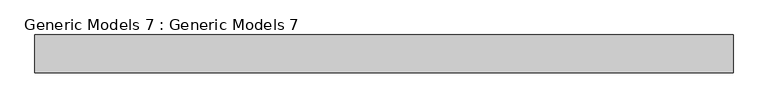
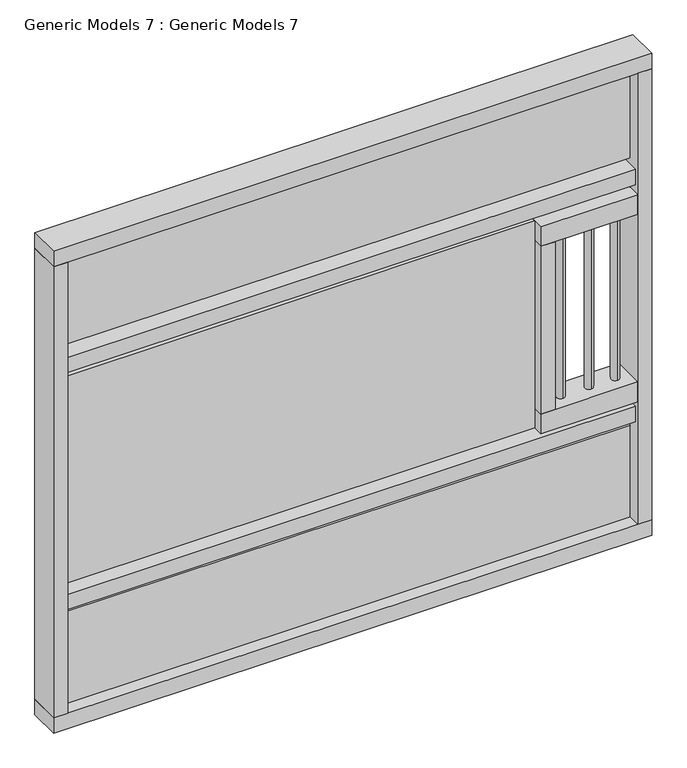
"""IFC4 building model written with IfcOpenShell, lengths in millimetres: proxy geometry, Generic Models 7 : Generic Models 7."""

from ifc_helpers import new_model, si_unit, point, frame, frame_2d, origin, place, context, project, spatial, polyline, circle_curve, trimmed, segment, composite_curve, outline, extrude, source, transform, mapped, element, save


def generic_models_7_generic_models_7_8565f2f4(model_context):
    return source(origin(), model_context, "Body", "SweptSolid", [
        extrude(outline(polyline([(-17469.9847028, -5427.8893448), (-17469.9847028, -5389.7874709), (-15982.9527072, -5389.7874709), (-15982.9527072, -5427.8893448), (-17469.9847028, -5427.8893448)])), frame((0.0, 0.0, 951.477172), z_axis=(0.0, 0.0, 1.0), x_axis=(1.0, 0.0, 0.0)), (0.0, 0.0, 1.0), 687.4014722),
        extrude(outline(composite_curve([segment(trimmed(circle_curve(frame_2d((-15722.0297157, -5413.1272599)), 12.7), [point((-15722.0297157, -5400.4272599))], [point((-15722.0297157, -5425.8272599))], False, "CARTESIAN"), True, "CONTINUOUS"), segment(trimmed(circle_curve(frame_2d((-15722.0297157, -5413.1272599)), 12.7), [point((-15722.0297157, -5425.8272599))], [point((-15722.0297157, -5400.4272599))], False, "CARTESIAN"), True, "CONTINUOUS")], self_intersect=False)), frame((0.0, 0.0, 1016.5786442), z_axis=(0.0, 0.0, 1.0), x_axis=(1.0, 0.0, 0.0)), (0.0, 0.0, 1.0), 564.5713558),
        extrude(outline(composite_curve([segment(trimmed(circle_curve(frame_2d((-15804.5797157, -5413.1272599)), 12.7), [point((-15804.5797157, -5400.4272599))], [point((-15804.5797157, -5425.8272599))], False, "CARTESIAN"), True, "CONTINUOUS"), segment(trimmed(circle_curve(frame_2d((-15804.5797157, -5413.1272599)), 12.7), [point((-15804.5797157, -5425.8272599))], [point((-15804.5797157, -5400.4272599))], False, "CARTESIAN"), True, "CONTINUOUS")], self_intersect=False)), frame((0.0, 0.0, 1016.5786442), z_axis=(0.0, 0.0, 1.0), x_axis=(1.0, 0.0, 0.0)), (0.0, 0.0, 1.0), 564.5713558),
        extrude(outline(composite_curve([segment(trimmed(circle_curve(frame_2d((-15893.4797157, -5413.1272599)), 12.7), [point((-15893.4797157, -5400.4272599))], [point((-15893.4797157, -5425.8272599))], False, "CARTESIAN"), True, "CONTINUOUS"), segment(trimmed(circle_curve(frame_2d((-15893.4797157, -5413.1272599)), 12.7), [point((-15893.4797157, -5425.8272599))], [point((-15893.4797157, -5400.4272599))], False, "CARTESIAN"), True, "CONTINUOUS")], self_intersect=False)), frame((0.0, 0.0, 1016.5786442), z_axis=(0.0, 0.0, 1.0), x_axis=(1.0, 0.0, 0.0)), (0.0, 0.0, 1.0), 564.5713558),
        extrude(outline(polyline([(-15982.9527072, -5358.3027976), (-15937.0252003, -5358.3027976), (-15937.0252003, -5459.9027976), (-15982.9527072, -5459.9027976), (-15982.9527072, -5358.3027976)])), frame((0.0, 0.0, 1016.5786442), z_axis=(0.0, 0.0, 1.0), x_axis=(1.0, 0.0, 0.0)), (0.0, 0.0, 1.0), 557.1985278),
        extrude(outline(polyline([(-15982.9527072, -5459.9027976), (-15982.9527072, -5358.3027976), (-15678.1527072, -5358.3027976), (-15678.1527072, -5459.9027976), (-15982.9527072, -5459.9027976)])), frame((0.0, 0.0, 1573.777172), z_axis=(0.0, 0.0, 1.0), x_axis=(1.0, 0.0, 0.0)), (0.0, 0.0, 1.0), 65.1014722),
        extrude(outline(polyline([(-15982.9527072, -5459.9027976), (-15982.9527072, -5358.3027976), (-15678.1527072, -5358.3027976), (-15678.1527072, -5459.9027976), (-15982.9527072, -5459.9027976)])), frame((0.0, 0.0, 951.477172), z_axis=(0.0, 0.0, 1.0), x_axis=(1.0, 0.0, 0.0)), (0.0, 0.0, 1.0), 65.1014722),
        extrude(outline(polyline([(-17469.9847028, -5447.389066), (-17469.9847028, -5371.189066), (-15678.1527072, -5371.189066), (-15678.1527072, -5447.389066), (-17469.9847028, -5447.389066)])), frame((0.0, 0.0, 1664.92529), z_axis=(0.0, 0.0, 1.0), x_axis=(1.0, 0.0, 0.0)), (0.0, 0.0, 1.0), 50.8),
        extrude(outline(polyline([(-17469.9847028, -5447.389066), (-17469.9847028, -5371.189066), (-15678.1527072, -5371.189066), (-15678.1527072, -5447.389066), (-17469.9847028, -5447.389066)])), frame((0.0, 0.0, 877.52529), z_axis=(0.0, 0.0, 1.0), x_axis=(1.0, 0.0, 0.0)), (0.0, 0.0, 1.0), 50.8),
        extrude(outline(polyline([(-17469.9847028, -5418.658566), (-17469.9847028, -5393.258566), (-15678.1527072, -5393.258566), (-15678.1527072, -5418.658566), (-17469.9847028, -5418.658566)])), frame((0.0, 0.0, 1737.2452447), z_axis=(0.0, 0.0, 1.0), x_axis=(1.0, 0.0, 0.0)), (0.0, 0.0, 1.0), 304.8),
        extrude(outline(polyline([(-17469.9847028, -5418.658566), (-17469.9847028, -5393.258566), (-15678.1527072, -5393.258566), (-15678.1527072, -5418.658566), (-17469.9847028, -5418.658566)])), frame((0.0, 0.0, 543.4452447), z_axis=(0.0, 0.0, 1.0), x_axis=(1.0, 0.0, 0.0)), (0.0, 0.0, 1.0), 304.8),
        extrude(outline(polyline([(-15634.268705, -5358.3027976), (-15634.268705, -5459.9027976), (-15678.1527072, -5459.9027976), (-15678.1527072, -5358.3027976), (-15634.268705, -5358.3027976)])), frame((0.0, 0.0, 543.4452447), z_axis=(0.0, 0.0, 1.0), x_axis=(1.0, 0.0, 0.0)), (0.0, 0.0, 1.0), 1498.6),
        extrude(outline(polyline([(-17469.9847028, -5358.3027976), (-17469.9847028, -5459.9027976), (-17513.868705, -5459.9027976), (-17513.868705, -5358.3027976), (-17469.9847028, -5358.3027976)])), frame((0.0, 0.0, 543.4452447), z_axis=(0.0, 0.0, 1.0), x_axis=(1.0, 0.0, 0.0)), (0.0, 0.0, 1.0), 1498.6),
        extrude(outline(polyline([(-17513.868705, -5459.9027976), (-17513.868705, -5358.3027976), (-15634.268705, -5358.3027976), (-15634.268705, -5459.9027976), (-17513.868705, -5459.9027976)])), frame((0.0, 0.0, 492.6452447), z_axis=(0.0, 0.0, 1.0), x_axis=(1.0, 0.0, 0.0)), (0.0, 0.0, 1.0), 50.8),
        extrude(outline(polyline([(-17513.868705, -5459.9027976), (-17513.868705, -5358.3027976), (-15634.268705, -5358.3027976), (-15634.268705, -5459.9027976), (-17513.868705, -5459.9027976)])), frame((0.0, 0.0, 2042.0452447), z_axis=(0.0, 0.0, 1.0), x_axis=(1.0, 0.0, 0.0)), (0.0, 0.0, 1.0), 50.8),
    ])


if __name__ == "__main__":
    model = new_model("IFC4")
    model_context = context("Model", 3, world=origin())
    ifc_project = project(units=[si_unit("LENGTHUNIT", "METRE", prefix="MILLI")], contexts=[model_context])
    site = spatial("IfcSite", under=ifc_project)
    building = spatial("IfcBuilding", under=site)
    placement = place(None, origin())
    generic_models_7_generic_models_7_shape = generic_models_7_generic_models_7_8565f2f4(model_context)
    element("IfcBuildingElementProxy", 1, Name="Generic Models 7 : Generic Models 7", ObjectType="Generic Models 7 : Generic Models 7", at=placement, inside=building, context=model_context, shape_type="MappedRepresentation", body=[
        mapped(generic_models_7_generic_models_7_shape, transform((0.0, 0.0, 0.0), x_axis=(1.0, 0.0, 0.0), y_axis=(0.0, 1.0, 0.0), z_axis=(0.0, 0.0, 1.0))),
    ])
    save(model, "model.ifc")

# Revit data of these elements
# Element 1 (IfcBuildingElementProxy, "Generic Models 7 : Generic Models 7")
#   Materials on its faces: "Damp-proofing", "Gypsum Wall Board", "Wood Planks"
# Materials
#   "Damp-proofing": class "Generic", colour RGB 17 17 17, transparency 0, Description = "Damp-proofing", Cost = 0
#   "Gypsum Wall Board": class "Generic", colour RGB 228 228 228, transparency 0, Description = "Gypsum Wall Board", Cost = 0
#   "Wood Planks": class "Wood", colour RGB 129 72 39, transparency 0, Description = "Physical material.", Cost = 0
